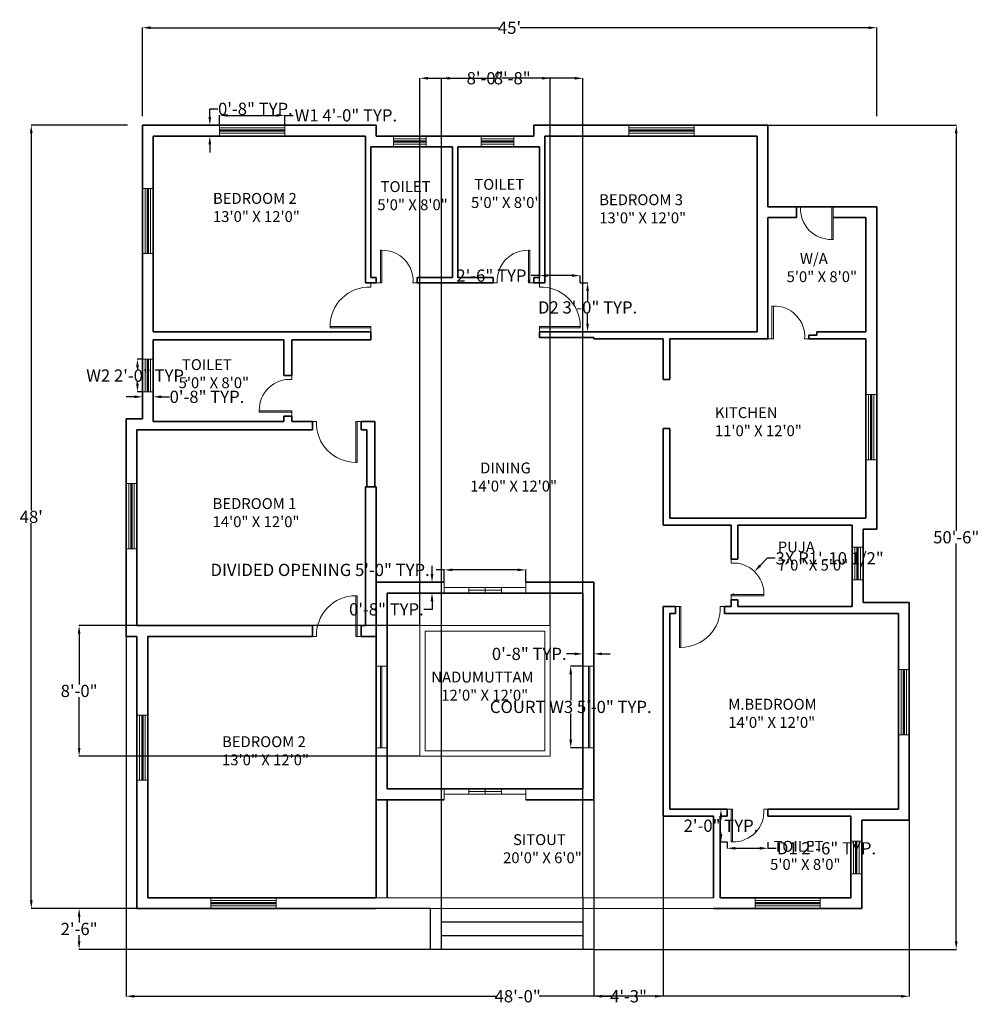
# Model space of a CAD drawing. Units: inches. Extents: x 1028 to 1734, y 196 to 920.
import ezdxf

# ---------------------------------------------------------------- set-up
doc = ezdxf.new("R2010")
doc.units = ezdxf.units.IN
doc.header["$MEASUREMENT"] = 0
for name, color, linetype, lineweight in [('A-ANNO-DIMS', 2, 'Continuous', 13), ('A-AREA-IDEN', 7, 'Continuous', 18), ('A-DOOR', 3, 'Continuous', 18), ('A-FLOR', 9, 'Continuous', 18), ('A-FLOR-STRS', 7, 'Continuous', 25), ('A-GLAZ', 4, 'Continuous', 15), ('A-WALL', 7, 'Continuous', 35)]:
    doc.layers.add(name, color=color, linetype=linetype, lineweight=lineweight)
doc.styles.get("Standard").update_dxf_attribs({"font": 'arial.ttf'})
doc.dimstyles.get("Standard").update_dxf_attribs({"dimtxt": 9, "dimasz": 6, "dimexe": 0.18, "dimexo": 0.0625, "dimgap": 0.09, "dimtad": 0, "dimtih": 1, "dimtoh": 1, "dimdec": 0, "dimzin": 0, "dimdsep": 46, "dimlunit": 3, "dimtxsty": 'Standard', "dimcen": 0.09, "dimadec": 0, "dimazin": 0, "dimtfac": 1, "dimtdec": 0, "dimtofl": 0, "dimtmove": 0, "dimatfit": 3, "dimfxl": 1, "dimtolj": 1, "dimtzin": 0, "dimarcsym": 0})

# ---------------------------------------------------------------- blocks, each defined once
blk = doc.blocks.new('*D1')
at = {"layer": 'A-ANNO-DIMS', "color": 0, "lineweight": -2, "transparency": 16777216}
for p, q in [((1107.07, 842.37), (1036.17, 842.37)), ((1036.35, 836.37), (1036.35, 559.05)), ((1036.35, 272.37), (1036.35, 549.68)), ((1107.07, 266.37), (1036.17, 266.37))]:
    blk.add_line(p, q, dxfattribs=at)
at = {"layer": 'A-ANNO-DIMS', "color": 0, "transparency": 16777216}
for points in [[(1035.35, 836.37), (1037.35, 836.37), (1036.35, 842.37)], [(1035.35, 272.37), (1037.35, 272.37), (1036.35, 266.37)]]:
    blk.add_solid(points, dxfattribs=at)
at = {"layer": 'Defpoints', "color": 0, "transparency": 16777216}
for p in [(1107.13, 842.37), (1036.35, 266.37), (1107.13, 266.37)]:
    blk.add_point(p, dxfattribs=at)
at = {"layer": 'A-ANNO-DIMS', "color": 0, "transparency": 16777216, "insert": (1036.35, 554.37), "char_height": 9, "attachment_point": 5}
blk.add_mtext("\\A1;48'", dxfattribs=at)
blk = doc.blocks.new('*D2')
at = {"layer": 'A-ANNO-DIMS', "color": 0, "lineweight": -2, "transparency": 16777216}
for p, q in [((1118.04, 849.03), (1118.04, 914.2)), ((1124.04, 914.02), (1380.13, 914.02)), ((1652.04, 914.02), (1395.95, 914.02)), ((1658.04, 849.03), (1658.04, 914.2))]:
    blk.add_line(p, q, dxfattribs=at)
at = {"layer": 'A-ANNO-DIMS', "color": 0, "transparency": 16777216}
for points in [[(1124.04, 915.02), (1124.04, 913.02), (1118.04, 914.02)], [(1652.04, 915.02), (1652.04, 913.02), (1658.04, 914.02)]]:
    blk.add_solid(points, dxfattribs=at)
at = {"layer": 'Defpoints', "color": 0, "transparency": 16777216}
for p in [(1658.04, 914.02), (1118.04, 848.97), (1658.04, 848.97)]:
    blk.add_point(p, dxfattribs=at)
at = {"layer": 'A-ANNO-DIMS', "color": 0, "transparency": 16777216, "insert": (1388.04, 914.02), "char_height": 9, "attachment_point": 5}
blk.add_mtext("\\A1;45'", dxfattribs=at)
blk = doc.blocks.new('DOOR-SWING-30IN')
blk.add_lwpolyline([(0, 30), (3, 30), (3, 0), (4, 0, 0.424176), (33, 30), (36, 30)], format="xyb")
blk.add_lwpolyline([(4, 0), (4, 30), (3, 30)])
blk = doc.blocks.new('DOOR-SWING-24IN')
for p, q in [((0, 27), (0, 30)), ((0, 3), (24, 3)), ((0, 3), (0, 0)), ((24, 3), (24, 4))]:
    blk.add_line(p, q)
blk.add_lwpolyline([(24, 4), (0, 4), (0, 3)])
blk.add_arc((1.62, 4.67), 22.39, 358.27839, 94.15936)
blk = doc.blocks.new('WIN-48IN')
for p, q in [((0, 8), (0, 0)), ((48, 8), (48, 0)), ((48, 6), (0, 6)), ((48, 4.5), (0, 4.5)), ((48, 4), (0, 4)), ((48, 3.5), (0, 3.5)), ((48, 2), (0, 2))]:
    blk.add_line(p, q)
blk = doc.blocks.new('WIN-24IN')
for p, q in [((0, 0), (0, 8)), ((24, 0), (24, 8)), ((0, 6), (24, 6)), ((0, 4.5), (24, 4.5)), ((0, 4), (24, 4)), ((0, 3.5), (24, 3.5)), ((0, 2), (24, 2))]:
    blk.add_line(p, q)
blk = doc.blocks.new('WIN-COURT-60IN')
for p, q in [((0, 60), (8, 60)), ((3, 60), (3, 0)), ((4, 60), (4, 0)), ((0, 0), (8, 0))]:
    blk.add_line(p, q)
blk = doc.blocks.new('OPENING-COURT-DIVIDED-60IN')
for p, q in [((0, 8), (0, 0)), ((18, 8), (18, 4)), ((30, 8), (30, 4)), ((42, 8), (42, 4)), ((60, 8), (60, 0)), ((0, 4), (60, 4)), ((18, 6), (42, 6))]:
    blk.add_line(p, q)
blk = doc.blocks.new('*D9')
at = {"layer": 'A-ANNO-DIMS', "color": 0, "lineweight": -2, "transparency": 16777216}
for p, q in [((1174.84, 842.43), (1174.84, 849.75)), ((1180.84, 849.57), (1216.84, 849.57)), ((1222.84, 842.43), (1222.84, 849.75)), ((1222.84, 849.57), (1228.84, 849.57))]:
    blk.add_line(p, q, dxfattribs=at)
at = {"layer": 'A-ANNO-DIMS', "color": 0, "transparency": 16777216}
for points in [[(1180.84, 850.57), (1180.84, 848.57), (1174.84, 849.57)], [(1216.84, 850.57), (1216.84, 848.57), (1222.84, 849.57)]]:
    blk.add_solid(points, dxfattribs=at)
at = {"layer": 'Defpoints', "color": 0, "transparency": 16777216}
for p in [(1222.84, 849.57), (1174.84, 842.37), (1222.84, 842.37)]:
    blk.add_point(p, dxfattribs=at)
at = {"layer": 'A-ANNO-DIMS', "color": 0, "transparency": 16777216, "insert": (1267.72, 849.57), "char_height": 9, "attachment_point": 5}
blk.add_mtext('\\A1;W1 4\'-0" TYP.', dxfattribs=at)
blk = doc.blocks.new('*D10')
at = {"layer": 'A-ANNO-DIMS', "color": 0, "lineweight": -2, "transparency": 16777216}
for p, q in [((1167.64, 848.37), (1167.64, 854.37)), ((1167.64, 854.37), (1173.64, 854.37)), ((1174.78, 842.37), (1167.46, 842.37)), ((1174.78, 834.37), (1167.46, 834.37)), ((1167.64, 828.37), (1167.64, 822.37))]:
    blk.add_line(p, q, dxfattribs=at)
at = {"layer": 'A-ANNO-DIMS', "color": 0, "transparency": 16777216}
for points in [[(1166.64, 848.37), (1168.64, 848.37), (1167.64, 842.37)], [(1166.64, 828.37), (1168.64, 828.37), (1167.64, 834.37)]]:
    blk.add_solid(points, dxfattribs=at)
at = {"layer": 'Defpoints', "color": 0, "transparency": 16777216}
for p in [(1167.64, 842.37), (1174.84, 842.37), (1174.84, 834.37)]:
    blk.add_point(p, dxfattribs=at)
at = {"layer": 'A-ANNO-DIMS', "color": 0, "transparency": 16777216, "insert": (1201.16, 854.37), "char_height": 9, "attachment_point": 5}
blk.add_mtext('\\A1;0\'-8" TYP.', dxfattribs=at)
blk = doc.blocks.new('*D11')
at = {"layer": 'A-ANNO-DIMS', "color": 0, "lineweight": -2, "transparency": 16777216}
for p, q in [((1117.98, 670.24), (1114.26, 670.24)), ((1114.44, 664.24), (1114.44, 662.93)), ((1114.44, 652.24), (1114.44, 653.56)), ((1117.98, 646.24), (1114.26, 646.24))]:
    blk.add_line(p, q, dxfattribs=at)
at = {"layer": 'A-ANNO-DIMS', "color": 0, "transparency": 16777216}
for points in [[(1113.44, 664.24), (1115.44, 664.24), (1114.44, 670.24)], [(1113.44, 652.24), (1115.44, 652.24), (1114.44, 646.24)]]:
    blk.add_solid(points, dxfattribs=at)
at = {"layer": 'Defpoints', "color": 0, "transparency": 16777216}
for p in [(1118.04, 670.24), (1114.44, 646.24), (1118.04, 646.24)]:
    blk.add_point(p, dxfattribs=at)
at = {"layer": 'A-ANNO-DIMS', "color": 0, "transparency": 16777216, "insert": (1114.44, 658.24), "char_height": 9, "attachment_point": 5}
blk.add_mtext('\\A1;W2 2\'-0" TYP.', dxfattribs=at)
blk = doc.blocks.new('*D12')
at = {"layer": 'A-ANNO-DIMS', "color": 0, "lineweight": -2, "transparency": 16777216}
for p, q in [((1118.04, 646.18), (1118.04, 642.46)), ((1126.04, 646.18), (1126.04, 642.46)), ((1112.04, 642.64), (1106.04, 642.64)), ((1132.04, 642.64), (1138.04, 642.64))]:
    blk.add_line(p, q, dxfattribs=at)
at = {"layer": 'A-ANNO-DIMS', "color": 0, "transparency": 16777216}
for points in [[(1112.04, 643.64), (1112.04, 641.64), (1118.04, 642.64)], [(1132.04, 643.64), (1132.04, 641.64), (1126.04, 642.64)]]:
    blk.add_solid(points, dxfattribs=at)
at = {"layer": 'Defpoints', "color": 0, "transparency": 16777216}
for p in [(1118.04, 646.24), (1126.04, 646.24), (1126.04, 642.64)]:
    blk.add_point(p, dxfattribs=at)
at = {"layer": 'A-ANNO-DIMS', "color": 0, "transparency": 16777216, "insert": (1165.56, 642.64), "char_height": 9, "attachment_point": 5}
blk.add_mtext('\\A1;0\'-8" TYP.', dxfattribs=at)
blk = doc.blocks.new('*D13')
at = {"layer": 'A-ANNO-DIMS', "color": 0, "lineweight": -2, "transparency": 16777216}
for p, q in [((1548.04, 315.11), (1548.04, 310.5)), ((1578.04, 315.11), (1578.04, 310.5)), ((1554.04, 310.68), (1572.04, 310.68)), ((1578.04, 310.68), (1584.04, 310.68))]:
    blk.add_line(p, q, dxfattribs=at)
at = {"layer": 'A-ANNO-DIMS', "color": 0, "transparency": 16777216}
for points in [[(1554.04, 311.68), (1554.04, 309.68), (1548.04, 310.68)], [(1572.04, 311.68), (1572.04, 309.68), (1578.04, 310.68)]]:
    blk.add_solid(points, dxfattribs=at)
at = {"layer": 'Defpoints', "color": 0, "transparency": 16777216}
for p in [(1548.04, 315.18), (1578.04, 315.18), (1578.04, 310.68)]:
    blk.add_point(p, dxfattribs=at)
at = {"layer": 'A-ANNO-DIMS', "color": 0, "transparency": 16777216, "insert": (1621.12, 310.68), "char_height": 9, "attachment_point": 5}
blk.add_mtext('\\A1;D1 2\'-6" TYP.', dxfattribs=at)
blk = doc.blocks.new('*D14')
at = {"layer": 'A-ANNO-DIMS', "color": 0, "lineweight": -2, "transparency": 16777216}
for p, q in [((1547.98, 339.37), (1543.36, 339.37)), ((1543.54, 333.37), (1543.54, 331.96)), ((1543.54, 321.18), (1543.54, 322.59)), ((1547.98, 315.18), (1543.36, 315.18))]:
    blk.add_line(p, q, dxfattribs=at)
at = {"layer": 'A-ANNO-DIMS', "color": 0, "transparency": 16777216}
for points in [[(1542.54, 333.37), (1544.54, 333.37), (1543.54, 339.37)], [(1542.54, 321.18), (1544.54, 321.18), (1543.54, 315.18)]]:
    blk.add_solid(points, dxfattribs=at)
at = {"layer": 'Defpoints', "color": 0, "transparency": 16777216}
for p in [(1548.04, 339.37), (1543.54, 315.18), (1548.04, 315.18)]:
    blk.add_point(p, dxfattribs=at)
at = {"layer": 'A-ANNO-DIMS', "color": 0, "transparency": 16777216, "insert": (1543.54, 327.27), "char_height": 9, "attachment_point": 5}
blk.add_mtext('\\A1;2\'-0" TYP.', dxfattribs=at)
blk = doc.blocks.new('*D15')
at = {"layer": 'A-ANNO-DIMS', "color": 0, "lineweight": -2, "transparency": 16777216}
for p, q in [((1440.1, 726.37), (1445.62, 726.37)), ((1445.44, 720.37), (1445.44, 713.06)), ((1445.44, 696.37), (1445.44, 703.68)), ((1440.1, 690.37), (1445.62, 690.37))]:
    blk.add_line(p, q, dxfattribs=at)
at = {"layer": 'A-ANNO-DIMS', "color": 0, "transparency": 16777216}
for points in [[(1444.44, 720.37), (1446.44, 720.37), (1445.44, 726.37)], [(1444.44, 696.37), (1446.44, 696.37), (1445.44, 690.37)]]:
    blk.add_solid(points, dxfattribs=at)
at = {"layer": 'Defpoints', "color": 0, "transparency": 16777216}
for p in [(1440.04, 726.37), (1445.44, 726.37), (1440.04, 690.37)]:
    blk.add_point(p, dxfattribs=at)
at = {"layer": 'A-ANNO-DIMS', "color": 0, "transparency": 16777216, "insert": (1445.44, 708.37), "char_height": 9, "attachment_point": 5}
blk.add_mtext('\\A1;D2 3\'-0" TYP.', dxfattribs=at)
blk = doc.blocks.new('*D16')
at = {"layer": 'A-ANNO-DIMS', "color": 0, "lineweight": -2, "transparency": 16777216}
for p, q in [((1410.04, 731.77), (1404.04, 731.77)), ((1410.04, 726.43), (1410.04, 731.95)), ((1434.04, 731.77), (1416.04, 731.77)), ((1440.04, 726.43), (1440.04, 731.95))]:
    blk.add_line(p, q, dxfattribs=at)
at = {"layer": 'A-ANNO-DIMS', "color": 0, "transparency": 16777216}
for points in [[(1416.04, 732.77), (1416.04, 730.77), (1410.04, 731.77)], [(1434.04, 732.77), (1434.04, 730.77), (1440.04, 731.77)]]:
    blk.add_solid(points, dxfattribs=at)
at = {"layer": 'Defpoints', "color": 0, "transparency": 16777216}
for p in [(1410.04, 731.77), (1410.04, 726.37), (1440.04, 726.37)]:
    blk.add_point(p, dxfattribs=at)
at = {"layer": 'A-ANNO-DIMS', "color": 0, "transparency": 16777216, "insert": (1376.44, 731.77), "char_height": 9, "attachment_point": 5}
blk.add_mtext('\\A1;2\'-6" TYP.', dxfattribs=at)
blk = doc.blocks.new('*D17')
at = {"layer": 'A-ANNO-DIMS', "color": 0, "lineweight": -2, "transparency": 16777216}
for p, q in [((1441.98, 444.63), (1432.86, 444.63)), ((1433.04, 438.63), (1433.04, 419.38)), ((1433.04, 390.63), (1433.04, 409.88)), ((1441.98, 384.63), (1432.86, 384.63))]:
    blk.add_line(p, q, dxfattribs=at)
at = {"layer": 'A-ANNO-DIMS', "color": 0, "transparency": 16777216}
for points in [[(1432.04, 438.63), (1434.04, 438.63), (1433.04, 444.63)], [(1432.04, 390.63), (1434.04, 390.63), (1433.04, 384.63)]]:
    blk.add_solid(points, dxfattribs=at)
at = {"layer": 'Defpoints', "color": 0, "transparency": 16777216}
for p in [(1442.04, 444.63), (1433.04, 384.63), (1442.04, 384.63)]:
    blk.add_point(p, dxfattribs=at)
at = {"layer": 'A-ANNO-DIMS', "color": 0, "transparency": 16777216, "insert": (1433.04, 414.63), "char_height": 9, "attachment_point": 5}
blk.add_mtext('\\A1;COURT W3 5\'-0" TYP.', dxfattribs=at)
blk = doc.blocks.new('*D18')
at = {"layer": 'A-ANNO-DIMS', "color": 0, "lineweight": -2, "transparency": 16777216}
for p, q in [((1436.04, 453.63), (1430.04, 453.63)), ((1442.04, 444.7), (1442.04, 453.81)), ((1450.04, 444.7), (1450.04, 453.81)), ((1456.04, 453.63), (1462.04, 453.63))]:
    blk.add_line(p, q, dxfattribs=at)
at = {"layer": 'A-ANNO-DIMS', "color": 0, "transparency": 16777216}
for points in [[(1436.04, 454.63), (1436.04, 452.63), (1442.04, 453.63)], [(1456.04, 454.63), (1456.04, 452.63), (1450.04, 453.63)]]:
    blk.add_solid(points, dxfattribs=at)
at = {"layer": 'Defpoints', "color": 0, "transparency": 16777216}
for p in [(1442.04, 453.63), (1442.04, 444.63), (1450.04, 444.63)]:
    blk.add_point(p, dxfattribs=at)
at = {"layer": 'A-ANNO-DIMS', "color": 0, "transparency": 16777216, "insert": (1402.52, 453.63), "char_height": 9, "attachment_point": 5}
blk.add_mtext('\\A1;0\'-8" TYP.', dxfattribs=at)
blk = doc.blocks.new('*D19')
at = {"layer": 'A-ANNO-DIMS', "color": 0, "lineweight": -2, "transparency": 16777216}
for p, q in [((1340.04, 515.37), (1334.04, 515.37)), ((1340.04, 506.43), (1340.04, 515.55)), ((1394.04, 515.37), (1346.04, 515.37)), ((1400.04, 506.43), (1400.04, 515.55))]:
    blk.add_line(p, q, dxfattribs=at)
at = {"layer": 'A-ANNO-DIMS', "color": 0, "transparency": 16777216}
for points in [[(1346.04, 516.37), (1346.04, 514.37), (1340.04, 515.37)], [(1394.04, 516.37), (1394.04, 514.37), (1400.04, 515.37)]]:
    blk.add_solid(points, dxfattribs=at)
at = {"layer": 'Defpoints', "color": 0, "transparency": 16777216}
for p in [(1340.04, 515.37), (1340.04, 506.37), (1400.04, 506.37)]:
    blk.add_point(p, dxfattribs=at)
at = {"layer": 'A-ANNO-DIMS', "color": 0, "transparency": 16777216, "insert": (1248.76, 515.37), "char_height": 9, "attachment_point": 5}
blk.add_mtext('\\A1;DIVIDED OPENING 5\'-0" TYP.', dxfattribs=at)
blk = doc.blocks.new('*D20')
at = {"layer": 'A-ANNO-DIMS', "color": 0, "lineweight": -2, "transparency": 16777216}
for p, q in [((1331.04, 512.37), (1331.04, 518.37)), ((1339.98, 506.37), (1330.86, 506.37)), ((1339.98, 498.37), (1330.86, 498.37)), ((1331.04, 492.37), (1331.04, 486.37)), ((1331.04, 486.37), (1325.04, 486.37))]:
    blk.add_line(p, q, dxfattribs=at)
at = {"layer": 'A-ANNO-DIMS', "color": 0, "transparency": 16777216}
for points in [[(1330.04, 512.37), (1332.04, 512.37), (1331.04, 506.37)], [(1330.04, 492.37), (1332.04, 492.37), (1331.04, 498.37)]]:
    blk.add_solid(points, dxfattribs=at)
at = {"layer": 'Defpoints', "color": 0, "transparency": 16777216}
for p in [(1340.04, 506.37), (1331.04, 498.37), (1340.04, 498.37)]:
    blk.add_point(p, dxfattribs=at)
at = {"layer": 'A-ANNO-DIMS', "color": 0, "transparency": 16777216, "insert": (1297.52, 486.37), "char_height": 9, "attachment_point": 5}
blk.add_mtext('\\A1;0\'-8" TYP.', dxfattribs=at)
blk = doc.blocks.new('*D21')
at = {"layer": 'A-ANNO-DIMS', "color": 0, "lineweight": -2, "transparency": 16777216}
for p, q in [((1106.04, 466.31), (1106.04, 201.69)), ((1682.04, 331.31), (1682.04, 201.69)), ((1112.04, 201.87), (1378.31, 201.87)), ((1676.04, 201.87), (1409.77, 201.87))]:
    blk.add_line(p, q, dxfattribs=at)
at = {"layer": 'A-ANNO-DIMS', "color": 0, "transparency": 16777216}
for points in [[(1112.04, 202.87), (1112.04, 200.87), (1106.04, 201.87)], [(1676.04, 202.87), (1676.04, 200.87), (1682.04, 201.87)]]:
    blk.add_solid(points, dxfattribs=at)
at = {"layer": 'Defpoints', "color": 0, "transparency": 16777216}
for p in [(1106.04, 466.37), (1682.04, 331.37), (1682.04, 201.87)]:
    blk.add_point(p, dxfattribs=at)
at = {"layer": 'A-ANNO-DIMS', "color": 0, "transparency": 16777216, "insert": (1394.04, 201.87), "char_height": 9, "attachment_point": 5}
blk.add_mtext('\\A1;48\'-0"', dxfattribs=at)
blk = doc.blocks.new('*D22')
at = {"layer": 'A-ANNO-DIMS', "color": 0, "lineweight": -2, "transparency": 16777216}
for p, q in [((1578.1, 842.37), (1716.72, 842.37)), ((1716.54, 836.37), (1716.54, 544.05)), ((1716.54, 242.37), (1716.54, 534.68)), ((1450.1, 236.37), (1716.72, 236.37))]:
    blk.add_line(p, q, dxfattribs=at)
at = {"layer": 'A-ANNO-DIMS', "color": 0, "transparency": 16777216}
for points in [[(1715.54, 836.37), (1717.54, 836.37), (1716.54, 842.37)], [(1715.54, 242.37), (1717.54, 242.37), (1716.54, 236.37)]]:
    blk.add_solid(points, dxfattribs=at)
at = {"layer": 'Defpoints', "color": 0, "transparency": 16777216}
for p in [(1578.04, 842.37), (1450.04, 236.37), (1716.54, 236.37)]:
    blk.add_point(p, dxfattribs=at)
at = {"layer": 'A-ANNO-DIMS', "color": 0, "transparency": 16777216, "insert": (1716.54, 539.37), "char_height": 9, "attachment_point": 5}
blk.add_mtext('\\A1;50\'-6"', dxfattribs=at)
blk = doc.blocks.new('*D23')
at = {"layer": 'A-ANNO-DIMS', "color": 0, "lineweight": -2, "transparency": 16777216}
for p, q in [((1322.04, 474.43), (1322.04, 877.05)), ((1328.04, 876.87), (1357.98, 876.87)), ((1412.04, 876.87), (1382.1, 876.87)), ((1418.04, 474.43), (1418.04, 877.05))]:
    blk.add_line(p, q, dxfattribs=at)
at = {"layer": 'A-ANNO-DIMS', "color": 0, "transparency": 16777216}
for points in [[(1328.04, 877.87), (1328.04, 875.87), (1322.04, 876.87)], [(1412.04, 877.87), (1412.04, 875.87), (1418.04, 876.87)]]:
    blk.add_solid(points, dxfattribs=at)
at = {"layer": 'Defpoints', "color": 0, "transparency": 16777216}
for p in [(1418.04, 876.87), (1322.04, 474.37), (1418.04, 474.37)]:
    blk.add_point(p, dxfattribs=at)
at = {"layer": 'A-ANNO-DIMS', "color": 0, "transparency": 16777216, "insert": (1370.04, 876.87), "char_height": 9, "attachment_point": 5}
blk.add_mtext('\\A1;8\'-0"', dxfattribs=at)
blk = doc.blocks.new('*D24')
at = {"layer": 'A-ANNO-DIMS', "color": 0, "lineweight": -2, "transparency": 16777216}
for p, q in [((1321.98, 474.37), (1071.36, 474.37)), ((1071.54, 468.37), (1071.54, 431.05)), ((1071.54, 384.37), (1071.54, 421.68)), ((1321.98, 378.37), (1071.36, 378.37))]:
    blk.add_line(p, q, dxfattribs=at)
at = {"layer": 'A-ANNO-DIMS', "color": 0, "transparency": 16777216}
for points in [[(1070.54, 468.37), (1072.54, 468.37), (1071.54, 474.37)], [(1070.54, 384.37), (1072.54, 384.37), (1071.54, 378.37)]]:
    blk.add_solid(points, dxfattribs=at)
at = {"layer": 'Defpoints', "color": 0, "transparency": 16777216}
for p in [(1322.04, 474.37), (1071.54, 378.37), (1322.04, 378.37)]:
    blk.add_point(p, dxfattribs=at)
at = {"layer": 'A-ANNO-DIMS', "color": 0, "transparency": 16777216, "insert": (1071.54, 426.37), "char_height": 9, "attachment_point": 5}
blk.add_mtext('\\A1;8\'-0"', dxfattribs=at)
blk = doc.blocks.new('*D25')
at = {"layer": 'A-ANNO-DIMS', "color": 0, "lineweight": -2, "transparency": 16777216}
for p, q in [((1338.04, 274.43), (1338.04, 877.05)), ((1344.04, 876.87), (1377.98, 876.87)), ((1436.04, 876.87), (1402.1, 876.87)), ((1442.04, 274.43), (1442.04, 877.05))]:
    blk.add_line(p, q, dxfattribs=at)
at = {"layer": 'A-ANNO-DIMS', "color": 0, "transparency": 16777216}
for points in [[(1344.04, 877.87), (1344.04, 875.87), (1338.04, 876.87)], [(1436.04, 877.87), (1436.04, 875.87), (1442.04, 876.87)]]:
    blk.add_solid(points, dxfattribs=at)
at = {"layer": 'Defpoints', "color": 0, "transparency": 16777216}
for p in [(1338.04, 876.87), (1338.04, 274.37), (1442.04, 274.37)]:
    blk.add_point(p, dxfattribs=at)
at = {"layer": 'A-ANNO-DIMS', "color": 0, "transparency": 16777216, "insert": (1390.04, 876.87), "char_height": 9, "attachment_point": 5}
blk.add_mtext('\\A1;8\'-8"', dxfattribs=at)
blk = doc.blocks.new('*D26')
at = {"layer": 'A-ANNO-DIMS', "color": 0, "lineweight": -2, "transparency": 16777216}
for p, q in [((1329.98, 266.37), (1071.36, 266.37)), ((1071.54, 260.37), (1071.54, 256.05)), ((1071.54, 242.37), (1071.54, 246.68)), ((1329.98, 236.37), (1071.36, 236.37))]:
    blk.add_line(p, q, dxfattribs=at)
at = {"layer": 'A-ANNO-DIMS', "color": 0, "transparency": 16777216}
for points in [[(1070.54, 260.37), (1072.54, 260.37), (1071.54, 266.37)], [(1070.54, 242.37), (1072.54, 242.37), (1071.54, 236.37)]]:
    blk.add_solid(points, dxfattribs=at)
at = {"layer": 'Defpoints', "color": 0, "transparency": 16777216}
for p in [(1330.04, 266.37), (1071.54, 236.37), (1330.04, 236.37)]:
    blk.add_point(p, dxfattribs=at)
at = {"layer": 'A-ANNO-DIMS', "color": 0, "transparency": 16777216, "insert": (1071.54, 251.37), "char_height": 9, "attachment_point": 5}
blk.add_mtext('\\A1;2\'-6"', dxfattribs=at)
blk = doc.blocks.new('*D27')
at = {"layer": 'A-ANNO-DIMS', "color": 0, "lineweight": -2, "transparency": 16777216}
for p, q in [((1450.04, 346.31), (1450.04, 201.69)), ((1501.04, 334.31), (1501.04, 201.69)), ((1456.04, 201.87), (1463.31, 201.87)), ((1495.04, 201.87), (1487.77, 201.87))]:
    blk.add_line(p, q, dxfattribs=at)
at = {"layer": 'A-ANNO-DIMS', "color": 0, "transparency": 16777216}
for points in [[(1456.04, 202.87), (1456.04, 200.87), (1450.04, 201.87)], [(1495.04, 202.87), (1495.04, 200.87), (1501.04, 201.87)]]:
    blk.add_solid(points, dxfattribs=at)
at = {"layer": 'Defpoints', "color": 0, "transparency": 16777216}
for p in [(1450.04, 346.37), (1501.04, 334.37), (1501.04, 201.87)]:
    blk.add_point(p, dxfattribs=at)
at = {"layer": 'A-ANNO-DIMS', "color": 0, "transparency": 16777216, "insert": (1475.54, 201.87), "char_height": 9, "attachment_point": 5}
blk.add_mtext('\\A1;4\'-3"', dxfattribs=at)
blk = doc.blocks.new('*D28')
at = {"layer": 'A-ANNO-DIMS', "color": 0, "lineweight": -2, "transparency": 16777216}
for p, q in [((1577.44, 523.9), (1572.3, 518.54)), ((1583.44, 523.9), (1577.44, 523.9)), ((1552.57, 498.04), (1552.75, 498.04)), ((1552.66, 497.95), (1552.66, 498.13))]:
    blk.add_line(p, q, dxfattribs=at)
at = {"layer": 'A-ANNO-DIMS', "color": 0, "transparency": 16777216}
blk.add_solid([(1571.58, 519.23), (1573.02, 517.84), (1568.15, 514.2)], dxfattribs=at)
at = {"layer": 'Defpoints', "color": 0, "transparency": 16777216}
for p in [(1568.15, 514.2), (1552.66, 498.04)]:
    blk.add_point(p, dxfattribs=at)
at = {"layer": 'A-ANNO-DIMS', "color": 0, "transparency": 16777216, "insert": (1623.45, 523.9), "char_height": 9, "attachment_point": 5}
blk.add_mtext('\\A1;3X R1\'-10 1/2"', dxfattribs=at)

msp = doc.modelspace()

# ---------------------------------------------------------------- linework, layer by layer
at = {"layer": 'A-FLOR'}
for p, q in [((1538.04, 274.37), (1290.04, 274.37)), ((1538.04, 266.37), (1290.04, 266.37))]:
    msp.add_line(p, q, dxfattribs=at)
for points in [[(1418.04, 474.37), (1322.04, 474.37), (1322.04, 378.37), (1418.04, 378.37)], [(1414.04, 470.37), (1326.04, 470.37), (1326.04, 382.37), (1414.04, 382.37)]]:
    msp.add_lwpolyline(points, close=True, dxfattribs=at)
at = {"layer": 'A-FLOR-STRS'}
for p, q in [((1338.04, 236.37), (1338.04, 274.37)), ((1442.04, 274.37), (1442.04, 236.37)), ((1330.04, 236.37), (1330.04, 266.37)), ((1450.04, 266.37), (1450.04, 236.37)), ((1442.04, 256.37), (1338.04, 256.37)), ((1442.04, 246.37), (1338.04, 246.37)), ((1450.04, 236.37), (1330.04, 236.37))]:
    msp.add_line(p, q, dxfattribs=at)
at = {"layer": 'A-WALL'}
for p, q in [((1118.04, 834.37), (1118.04, 842.37)), ((1118.04, 842.37), (1282.04, 842.37)), ((1282.04, 842.37), (1290.04, 842.37)), ((1290.04, 842.37), (1290.04, 834.37)), ((1414.04, 842.37), (1406.04, 842.37)), ((1406.04, 842.37), (1406.04, 834.37)), ((1578.04, 842.37), (1414.04, 842.37)), ((1578.04, 834.37), (1578.04, 842.37)), ((1118.04, 626.37), (1118.04, 834.37)), ((1126.04, 690.37), (1126.04, 834.37)), ((1126.04, 834.37), (1282.04, 834.37)), ((1282.04, 834.37), (1282.04, 726.37)), ((1290.04, 834.37), (1406.04, 834.37)), ((1414.04, 834.37), (1570.04, 834.37)), ((1414.04, 726.37), (1414.04, 834.37)), ((1570.04, 834.37), (1570.04, 690.37)), ((1578.04, 834.37), (1578.04, 782.37)), ((1286.04, 826.37), (1346.04, 826.37)), ((1286.04, 730.37), (1286.04, 826.37)), ((1346.04, 826.37), (1346.04, 730.37)), ((1350.04, 826.37), (1410.04, 826.37)), ((1350.04, 730.37), (1350.04, 826.37)), ((1410.04, 826.37), (1410.04, 730.37)), ((1658.04, 782.37), (1578.04, 782.37)), ((1599.04, 774.37), (1599.04, 782.37)), ((1658.04, 545.37), (1658.04, 782.37)), ((1578.04, 774.37), (1578.04, 690.37)), ((1599.04, 774.37), (1578.04, 774.37)), ((1650.04, 774.37), (1626.04, 774.37)), ((1650.04, 690.37), (1650.04, 774.37)), ((1286.04, 726.37), (1282.04, 726.37)), ((1290.04, 730.37), (1286.04, 730.37)), ((1290.04, 726.37), (1286.04, 726.37)), ((1290.04, 730.37), (1290.04, 726.37)), ((1346.04, 730.37), (1320.04, 730.37)), ((1320.04, 730.37), (1320.04, 726.37)), ((1376.04, 726.37), (1320.04, 726.37)), ((1376.04, 730.37), (1350.04, 730.37)), ((1376.04, 730.37), (1376.04, 726.37)), ((1410.04, 730.37), (1406.04, 730.37)), ((1406.04, 730.37), (1406.04, 726.37)), ((1410.04, 726.37), (1406.04, 726.37)), ((1410.04, 726.37), (1414.04, 726.37)), ((1282.04, 690.37), (1126.04, 690.37)), ((1282.04, 690.37), (1286.04, 690.37)), ((1286.04, 684.43), (1286.04, 690.37)), ((1410.04, 690.37), (1410.04, 686.37)), ((1414.04, 690.37), (1410.04, 690.37)), ((1570.04, 690.37), (1414.04, 690.37)), ((1578.04, 690.37), (1578.04, 685.37)), ((1608.04, 687.87), (1608.04, 685.37)), ((1614.04, 687.87), (1608.04, 687.87)), ((1614.04, 690.37), (1650.04, 690.37)), ((1614.04, 690.37), (1614.04, 687.87)), ((1126.04, 684.43), (1222.04, 684.43)), ((1126.04, 624.43), (1126.04, 684.43)), ((1222.04, 684.43), (1209.56, 684.43)), ((1222.04, 684.43), (1222.04, 658.43)), ((1222.04, 684.37), (1222.04, 676.51)), ((1286.04, 684.43), (1228.04, 684.43)), ((1228.04, 684.43), (1228.04, 658.43)), ((1410.04, 686.37), (1450.04, 686.37)), ((1450.04, 686.37), (1450.04, 685.37)), ((1501.04, 685.37), (1450.04, 685.37)), ((1501.04, 685.37), (1501.04, 655.37)), ((1506.04, 685.37), (1506.04, 655.37)), ((1570.04, 685.37), (1506.04, 685.37)), ((1578.04, 685.37), (1506.04, 685.37)), ((1650.04, 685.37), (1608.04, 685.37)), ((1650.04, 553.37), (1650.04, 685.37)), ((1222.04, 658.43), (1228.04, 658.43)), ((1501.04, 655.37), (1506.04, 655.37)), ((1106.04, 618.37), (1106.04, 626.37)), ((1106.04, 626.37), (1118.04, 626.37)), ((1222.04, 624.43), (1126.04, 624.43)), ((1221.98, 624.43), (1209.56, 624.43)), ((1221.98, 624.43), (1222.04, 624.43)), ((1222.04, 628.43), (1228.04, 628.43)), ((1222.04, 628.43), (1222.04, 624.43)), ((1228.04, 628.43), (1228.04, 624.43)), ((1228.04, 624.43), (1243.04, 624.43)), ((1243.04, 618.37), (1243.04, 624.43)), ((1279.04, 618.37), (1279.04, 624.43)), ((1279.04, 624.43), (1282.04, 624.43)), ((1282.04, 624.43), (1289.04, 624.43)), ((1289.04, 576.43), (1289.04, 624.43)), ((1106.04, 474.37), (1106.04, 618.37)), ((1114.04, 618.37), (1243.04, 618.37)), ((1114.04, 474.37), (1114.04, 618.37)), ((1279.04, 618.37), (1283.04, 618.37)), ((1283.04, 576.43), (1283.04, 618.37)), ((1501.04, 619.37), (1506.04, 619.37)), ((1501.04, 619.37), (1501.04, 548.37)), ((1506.04, 619.37), (1506.04, 553.37)), ((1282.04, 576.43), (1282.04, 474.37)), ((1282.04, 576.43), (1290.04, 576.43)), ((1290.04, 550.94), (1290.04, 576.43)), ((1290.04, 498.37), (1290.04, 550.94)), ((1506.04, 553.37), (1650.04, 553.37)), ((1501.04, 548.37), (1551.04, 548.37)), ((1551.04, 523.37), (1551.04, 548.37)), ((1556.04, 548.37), (1640.04, 548.37)), ((1556.04, 523.37), (1556.04, 548.37)), ((1640.04, 488.37), (1640.04, 548.37)), ((1648.04, 491.37), (1648.04, 545.37)), ((1648.04, 545.37), (1658.04, 545.37)), ((1556.04, 523.37), (1551.04, 523.37)), ((1290.04, 506.37), (1340.04, 506.37)), ((1400.04, 506.37), (1450.04, 506.37)), ((1450.04, 506.37), (1450.04, 346.37)), ((1290.04, 346.37), (1290.04, 498.37)), ((1298.04, 498.37), (1442.04, 498.37)), ((1298.04, 354.37), (1298.04, 498.37)), ((1442.04, 498.37), (1442.04, 354.37)), ((1551.04, 488.37), (1551.04, 493.37)), ((1556.04, 493.37), (1551.04, 493.37)), ((1556.04, 488.37), (1556.04, 493.37)), ((1298.04, 354.37), (1298.04, 490.37)), ((1501.04, 488.37), (1510.04, 488.37)), ((1501.04, 334.37), (1501.04, 488.37)), ((1510.04, 483.37), (1510.04, 488.37)), ((1546.04, 483.37), (1546.04, 488.37)), ((1546.04, 488.37), (1551.04, 488.37)), ((1556.04, 488.37), (1640.04, 488.37)), ((1682.04, 491.37), (1648.04, 491.37)), ((1682.04, 483.37), (1682.04, 491.37)), ((1506.04, 483.37), (1510.04, 483.37)), ((1506.04, 339.37), (1506.04, 483.37)), ((1546.04, 483.37), (1674.04, 483.37)), ((1674.04, 483.37), (1674.04, 339.37)), ((1682.04, 331.37), (1682.04, 483.37)), ((1106.04, 474.37), (1106.04, 466.37)), ((1243.04, 474.37), (1114.04, 474.37)), ((1243.04, 466.37), (1243.04, 474.37)), ((1282.04, 474.37), (1279.04, 474.37)), ((1279.04, 466.37), (1279.04, 474.37)), ((1106.04, 466.37), (1114.04, 466.37)), ((1114.04, 466.37), (1114.04, 266.37)), ((1122.04, 466.37), (1122.04, 274.37)), ((1243.04, 466.37), (1122.04, 466.37)), ((1290.04, 466.37), (1279.04, 466.37)), ((1442.04, 354.37), (1298.04, 354.37)), ((1290.04, 274.37), (1290.04, 346.37)), ((1340.04, 346.37), (1290.04, 346.37)), ((1298.04, 274.37), (1298.04, 346.37)), ((1450.04, 346.37), (1400.04, 346.37)), ((1538.04, 334.37), (1501.04, 334.37)), ((1506.04, 339.37), (1548.04, 339.37)), ((1538.04, 334.37), (1538.04, 274.37)), ((1543.04, 334.37), (1543.04, 274.37)), ((1548.04, 334.37), (1543.04, 334.37)), ((1548.04, 334.37), (1548.04, 339.37)), ((1578.04, 334.37), (1578.04, 339.37)), ((1578.04, 339.37), (1674.04, 339.37)), ((1639.04, 334.37), (1578.04, 334.37)), ((1639.04, 334.37), (1639.04, 274.37)), ((1647.04, 331.37), (1647.04, 266.37)), ((1647.04, 331.37), (1674.04, 331.37)), ((1674.04, 331.37), (1682.04, 331.37)), ((1122.04, 274.37), (1290.04, 274.37)), ((1543.04, 274.37), (1639.04, 274.37)), ((1114.04, 266.37), (1290.04, 266.37)), ((1538.04, 266.37), (1647.04, 266.37))]:
    msp.add_line(p, q, dxfattribs=at)

# ---------------------------------------------------------------- block references
at = {"layer": 'A-DOOR', "extrusion": (0, 0, -1), "zscale": -1}
for name, p, rotation in [('DOOR-SWING-24IN', (-1629.04, 782.37), 270.0000000000015), ('DOOR-SWING-24IN', (-1290.04, 726.37), 90.00000000000104), ('DOOR-SWING-30IN', (-1256.04, 690.37), 89.99999999999982), ('DOOR-SWING-24IN', (-1578.04, 685.37), 90.00000000000078)]:
    msp.add_blockref(name, p, dxfattribs=dict(at, rotation=rotation))
at = {"layer": 'A-DOOR'}
for name, p, rotation in [('DOOR-SWING-24IN', (1406.04, 726.37), 90.0000000000023), ('DOOR-SWING-30IN', (1440.04, 690.37), 89.99999999999945), ('DOOR-SWING-30IN', (1279.04, 496.37), 180), ('DOOR-SWING-24IN', (1548.04, 339.37), 270.0000000000016)]:
    msp.add_blockref(name, p, dxfattribs=dict(at, rotation=rotation))
at = {"layer": 'A-DOOR', "extrusion": (0, 0, -1), "zscale": -1}
for name, p in [('DOOR-SWING-24IN', (-1228.04, 628.43)), ('DOOR-SWING-30IN', (-1279.04, 594.43))]:
    msp.add_blockref(name, p, dxfattribs=at)
at = {"layer": 'A-DOOR'}
for name, p in [('DOOR-SWING-24IN', (1551.04, 493.37)), ('DOOR-SWING-30IN', (1510.04, 458.37))]:
    msp.add_blockref(name, p, dxfattribs=at)
at = {"layer": 'A-GLAZ'}
for name, p in [('WIN-48IN', (1174.84, 834.37)), ('WIN-48IN', (1475.74, 834.37)), ('WIN-24IN', (1302.63, 826.37)), ('WIN-24IN', (1367.09, 826.37)), ('WIN-COURT-60IN', (1290.04, 384.63)), ('OPENING-COURT-DIVIDED-60IN', (1340.04, 346.37)), ('WIN-48IN', (1168.42, 266.37)), ('WIN-48IN', (1568.6, 266.37))]:
    msp.add_blockref(name, p, dxfattribs=at)
for name, p, rotation in [('WIN-48IN', (1126.04, 747.92), 89.99999999999898), ('WIN-24IN', (1118.04, 670.24), 269.999999999999), ('WIN-48IN', (1658.04, 596.23), 89.99999999999947), ('WIN-48IN', (1114.04, 530.81), 89.99999999999895), ('WIN-24IN', (1640.04, 532.15), 269.9999999999978), ('OPENING-COURT-DIVIDED-60IN', (1400.04, 506.37), 180), ('WIN-COURT-60IN', (1450.04, 444.63), 180), ('WIN-48IN', (1682.04, 394.18), 89.99999999999955), ('WIN-48IN', (1122.04, 360.68), 89.99999999999905), ('WIN-24IN', (1639.04, 315.97), 269.999999999997)]:
    msp.add_blockref(name, p, dxfattribs=dict(at, rotation=rotation))

# ---------------------------------------------------------------- texts
at = {"layer": 'A-AREA-IDEN', "char_height": 8, "attachment_point": 1}
for s, insert in [(' TOILET\\P5\'0" X 8\'0"', (1290.83, 801.2)), (' TOILET\\P5\'0" X 8\'0"', (1359.72, 802.84)), ('BEDROOM 2\\P13\'0" X 12\'0"', (1169.98, 792.51)), ('BEDROOM 3\\P13\'0" X 12\'0"', (1454.01, 791.54)), ('    W/A\\P5\'0" X 8\'0"', (1591.8, 748.28)), (' TOILET\\P5\'0" X 8\'0"', (1144.71, 670.31)), ('KITCHEN\\P11\'0" X 12\'0"', (1539.1, 635)), ('   DINING\\P14\'0" X 12\'0"', (1359.12, 594.33)), ('BEDROOM 1\\P14\'0" X 12\'0"', (1169.69, 568.13)), ('PUJA\\P7\'0" X 5\'0"', (1585.29, 536.23)), ('NADUMUTTAM\\P   12\'0" X 12\'0"', (1330.54, 440.58)), ('M.BEDROOM \\P14\'0" X 12\'0"', (1548.91, 420.57)), ('BEDROOM 2\\P13\'0" X 12\'0"', (1176.66, 393.04)), ('   SITOUT\\P20\'0" X 6\'0"', (1383.32, 321.05)), (' TOILET\\P5\'0" X 8\'0"', (1579.66, 316.16))]:
    msp.add_mtext_dynamic_manual_height_columns(s, width=141.527, gutter_width=1, heights=[0], dxfattribs=dict(at, insert=insert))

# ---------------------------------------------------------------- dimensions: what is measured, and where the dimension line sits
at = {"layer": 'A-ANNO-DIMS'}
for base, p1, p2, override, picture, middle in [((1658.04, 914.02), (1118.04, 848.97), (1658.04, 848.97), {"dimclrd": 0, "dimclre": 0, "dimclrt": 0}, '*D2', (1388.04, 914.02)), ((1418.04, 876.87), (1322.04, 474.37), (1418.04, 474.37), {"dimdec": 1, "dimlfac": 1, "dimrnd": 0, "dimzin": 1, "dimdsep": 46, "dimlunit": 4, "dimfrac": 2}, '*D23', (1370.04, 876.87)), ((1338.04, 876.87), (1442.04, 274.37), (1338.04, 274.37), {"dimdec": 1, "dimlfac": 1, "dimrnd": 0, "dimzin": 1, "dimdsep": 46, "dimlunit": 4, "dimfrac": 2}, '*D25', (1390.04, 876.87)), ((1682.04, 201.87), (1106.04, 466.37), (1682.04, 331.37), {"dimdec": 1, "dimlfac": 1, "dimrnd": 0, "dimzin": 1, "dimdsep": 46, "dimlunit": 4, "dimfrac": 2}, '*D21', (1394.04, 201.87)), ((1501.04, 201.87), (1450.04, 346.37), (1501.04, 334.37), {"dimdec": 1, "dimlfac": 1, "dimrnd": 0, "dimzin": 1, "dimdsep": 46, "dimlunit": 4, "dimfrac": 2}, '*D27', (1475.54, 201.87))]:
    dim = msp.add_linear_dim(base=base, p1=p1, p2=p2, dimstyle='Standard', override=override, dxfattribs=at)
    dim.commit()
    dim.dimension.update_dxf_attribs({"geometry": picture, "text_midpoint": middle})
for base, p1, p2, text, picture, middle in [((1222.84, 849.57), (1174.84, 842.37), (1222.84, 842.37), 'W1 <> TYP.', '*D9', (1267.72, 849.57)), ((1126.04, 642.64), (1118.04, 646.24), (1126.04, 646.24), '<> TYP.', '*D12', (1165.56, 642.64))]:
    dim = msp.add_linear_dim(base=base, p1=p1, p2=p2, text=text, dimstyle='Standard', override={"dimdec": 1, "dimlfac": 1, "dimrnd": 0, "dimzin": 1, "dimdsep": 46, "dimlunit": 4, "dimfrac": 2}, dxfattribs=at)
    dim.commit()
    dim.dimension.update_dxf_attribs({"geometry": picture, "text_midpoint": middle})
for base, p1, p2, angle, text, picture, middle in [((1167.64, 842.37), (1174.84, 834.37), (1174.84, 842.37), 90, '<> TYP.', '*D10', (1201.16, 854.37)), ((1410.04, 731.77), (1440.04, 726.37), (1410.04, 726.37), 180, '<> TYP.', '*D16', (1376.44, 731.77)), ((1445.44, 726.37), (1440.04, 690.37), (1440.04, 726.37), 90, 'D2 <> TYP.', '*D15', (1445.44, 708.37)), ((1114.44, 646.24), (1118.04, 670.24), (1118.04, 646.24), 270, 'W2 <> TYP.', '*D11', (1114.44, 658.24)), ((1340.04, 515.37), (1400.04, 506.37), (1340.04, 506.37), 180, 'DIVIDED OPENING <> TYP.', '*D19', (1248.76, 515.37)), ((1331.04, 498.37), (1340.04, 506.37), (1340.04, 498.37), 270, '<> TYP.', '*D20', (1297.52, 486.37)), ((1442.04, 453.63), (1450.04, 444.63), (1442.04, 444.63), 180, '<> TYP.', '*D18', (1402.52, 453.63)), ((1433.04, 384.63), (1442.04, 444.63), (1442.04, 384.63), 270, 'COURT W3 <> TYP.', '*D17', (1433.04, 414.63)), ((1543.54, 315.18), (1548.04, 339.37), (1548.04, 315.18), 270, '<> TYP.', '*D14', (1543.54, 327.27)), ((1578.04, 310.68), (1548.04, 315.18), (1578.04, 315.18), 0, 'D1 <> TYP.', '*D13', (1621.12, 310.68))]:
    dim = msp.add_linear_dim(base=base, p1=p1, p2=p2, angle=angle, text=text, dimstyle='Standard', override={"dimdec": 1, "dimlfac": 1, "dimrnd": 0, "dimzin": 1, "dimdsep": 46, "dimlunit": 4, "dimfrac": 2}, dxfattribs=at)
    dim.commit()
    dim.dimension.update_dxf_attribs({"geometry": picture, "text_midpoint": middle})
for base, p1, p2, override, picture, middle in [((1036.35, 266.37), (1107.13, 842.37), (1107.13, 266.37), {"dimclrd": 0, "dimclre": 0, "dimclrt": 0}, '*D1', (1036.35, 554.37)), ((1716.54, 236.37), (1578.04, 842.37), (1450.04, 236.37), {"dimdec": 1, "dimlfac": 1, "dimrnd": 0, "dimzin": 1, "dimdsep": 46, "dimlunit": 4, "dimfrac": 2}, '*D22', (1716.54, 539.37)), ((1071.54, 378.37), (1322.04, 474.37), (1322.04, 378.37), {"dimdec": 1, "dimlfac": 1, "dimrnd": 0, "dimzin": 1, "dimdsep": 46, "dimlunit": 4, "dimfrac": 2}, '*D24', (1071.54, 426.37)), ((1071.54, 236.37), (1330.04, 266.37), (1330.04, 236.37), {"dimdec": 1, "dimlfac": 1, "dimrnd": 0, "dimzin": 1, "dimdsep": 46, "dimlunit": 4, "dimfrac": 2}, '*D26', (1071.54, 251.37))]:
    dim = msp.add_linear_dim(base=base, p1=p1, p2=p2, angle=90, dimstyle='Standard', override=override, dxfattribs=at)
    dim.commit()
    dim.dimension.update_dxf_attribs({"geometry": picture, "text_midpoint": middle})
dim = msp.add_radius_dim(center=(1552.66, 498.04), mpoint=(1568.15, 514.2), text='3X <>', dimstyle='Standard', override={"dimdec": 1, "dimlfac": 1, "dimrnd": 0, "dimzin": 1, "dimdsep": 46, "dimlunit": 4, "dimfrac": 2}, dxfattribs=at)
dim.commit()
dim.dimension.update_dxf_attribs({"geometry": '*D28', "text_midpoint": (1623.45, 523.9), "dimtype": 164})

doc.saveas('drawing.dxf')
